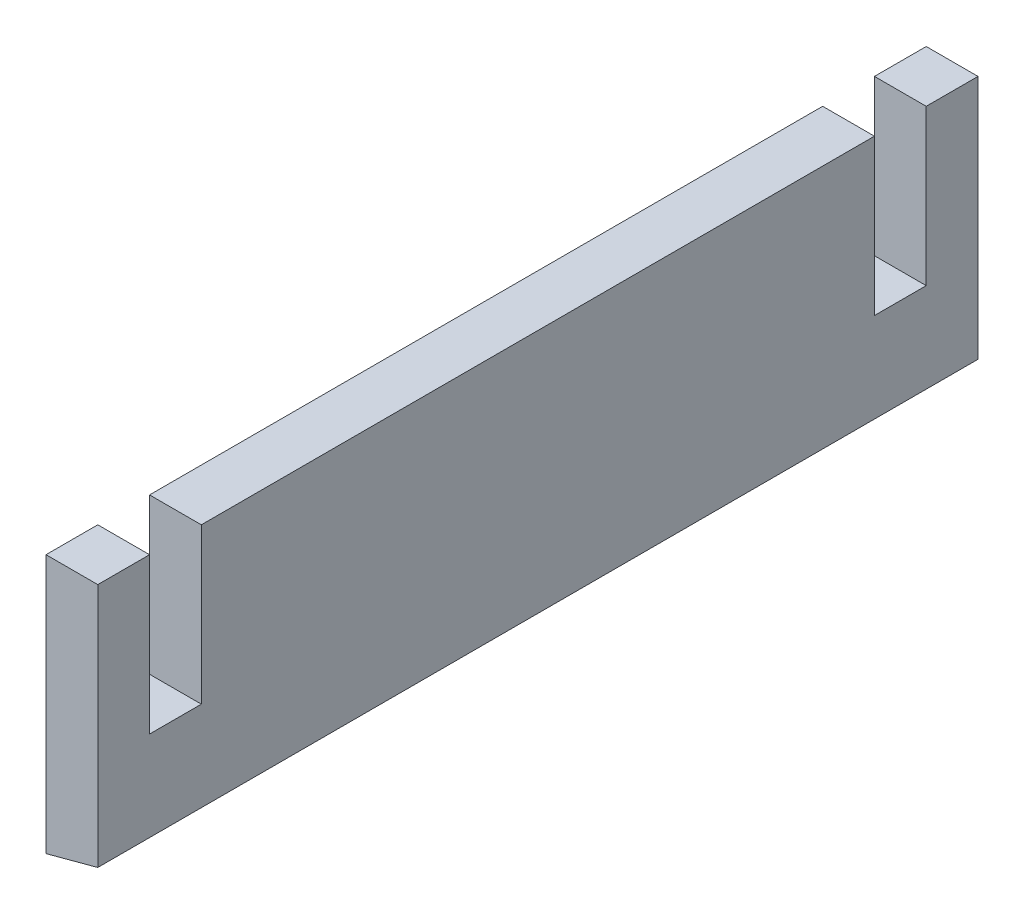
SolidWorks part; units mm, degrees
material "Plain Carbon Steel"
ref_plane "Front Plane" through (0, 0, 0) normal (0, 0, 1) x (1, 0, 0)
ref_plane "Top Plane" through (0, 0, 0) normal (0, 1, 0) x (1, 0, 0)
ref_plane "Right Plane" through (0, 0, 0) normal (1, 0, 0) x (0, 0, -1)
sketch "Step Plate Profile" plane through (0, 0, 0) normal (1, 0, 0) x (0, 0, -1)
  line L0 (0, 0) -> (170, 0)
  line L1 (170, 0) -> (170, 50)
  line L2 (170, 50) -> (160, 50)
  line L3 (160, 50) -> (160, 20)
  line L4 (160, 20) -> (150, 20)
  line L5 (150, 20) -> (150, 50)
  line L6 (150, 50) -> (20, 50)
  line L7 (20, 50) -> (20, 20)
  line L8 (20, 20) -> (10, 20)
  line L9 (10, 20) -> (10, 50)
  line L10 (10, 50) -> (0, 50)
  line L11 (0, 50) -> (0, 0)
  dimension "D1" = 170
  dimension "D2" = 10
  dimension "D3" = 10
  dimension "D4" = 10
  dimension "D5" = 10
  dimension "D6" = 30
  dimension "D7" = 30
  dimension "D8" = 50
extrude "Step Plate 10mm" add sketch "Step Plate Profile" along normal mid plane 10
draft "Draft 15deg" type of draft neutral plane draft angle 15 faces to draft 1 face at (0, 0, -85) neutral plane through (-5, 0, 0) neutral plane normal (-1, 0, 0) reverse direction yes parameters "D1"=15
